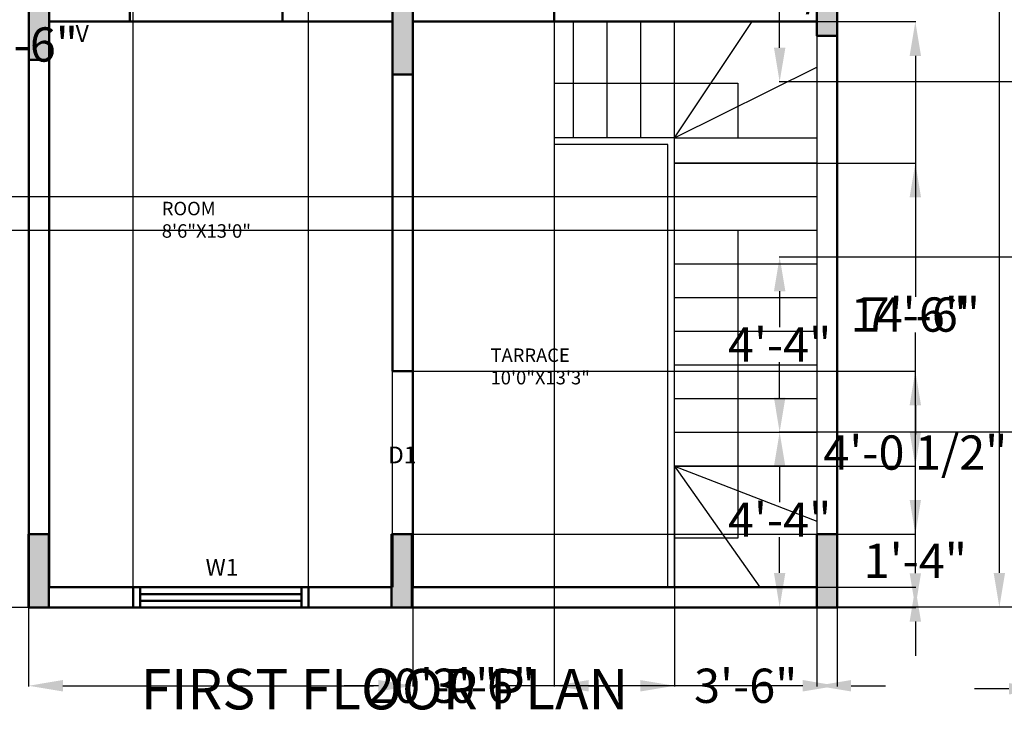
# Model space of a CAD drawing. Units: inches. Extents: x 21 to 3450, y 4 to 2137.
# Tile 3 of 14: x 2513 to 2805, y 1056 to 1261. Entities that reach past the tile are written whole.
import ezdxf

# ---------------------------------------------------------------- set-up
doc = ezdxf.new("R2010")
doc.units = ezdxf.units.IN
doc.header["$MEASUREMENT"] = 0
for name, color, linetype, lineweight in [('A-ANNO-DIMS', 2, 'Continuous', 18), ('A-ANNO-TEXT', 7, 'Continuous', 18), ('A-AREA-IDEN', 3, 'Continuous', 18), ('A-FLOR-STRS', 2, 'Continuous', 25), ('A-WALL', 7, 'Continuous', 50), ('A-WALL-PATT', 8, 'Continuous', 13)]:
    doc.layers.add(name, color=color, linetype=linetype, lineweight=lineweight)
doc.styles.get("Standard").update_dxf_attribs({"font": 'arial.ttf'})
doc.dimstyles.get("Standard").update_dxf_attribs({"dimtxt": 10.18, "dimasz": 10.18, "dimexe": 0.18, "dimexo": 0.0625, "dimgap": 0.09, "dimtad": 0, "dimtih": 1, "dimtoh": 1, "dimdec": 0, "dimzin": 0, "dimdsep": 46, "dimlunit": 3, "dimtxsty": 'Standard', "dimcen": 0.09, "dimadec": 0, "dimazin": 0, "dimtfac": 1, "dimtdec": 0, "dimtofl": 0, "dimtmove": 0, "dimatfit": 3, "dimfxl": 1, "dimtolj": 1, "dimtzin": 0, "dimarcsym": 0})

# ---------------------------------------------------------------- blocks, each defined once
blk = doc.blocks.new('*D8')
at = {"layer": 'A-ANNO-DIMS', "color": 0, "lineweight": -2, "transparency": 16777216}
for p, q in [((2816.85, 1506.81), (2803.73, 1506.81)), ((2803.91, 1496.63), (2803.91, 1302.07)), ((2803.91, 1096.92), (2803.91, 1291.48)), ((2999.5, 1086.74), (2803.73, 1086.74))]:
    blk.add_line(p, q, dxfattribs=at)
at = {"layer": 'A-ANNO-DIMS', "color": 0, "transparency": 16777216}
for points in [[(2802.22, 1496.63), (2805.61, 1496.63), (2803.91, 1506.81)], [(2802.22, 1096.92), (2805.61, 1096.92), (2803.91, 1086.74)]]:
    blk.add_solid(points, dxfattribs=at)
at = {"layer": 'Defpoints', "color": 0, "transparency": 16777216}
for p in [(2816.91, 1506.81), (2803.91, 1086.74), (2999.56, 1086.74)]:
    blk.add_point(p, dxfattribs=at)
at = {"layer": 'A-ANNO-DIMS', "color": 0, "transparency": 16777216, "insert": (2803.91, 1296.77), "char_height": 10.18, "attachment_point": 5}
blk.add_mtext("\\A1;35'", dxfattribs=at)
blk = doc.blocks.new('*D46')
at = {"layer": 'A-ANNO-DIMS', "color": 0, "lineweight": -2, "transparency": 16777216}
for p, q in [((2491.15, 1243.68), (2491.15, 1253.86)), ((2491.15, 1253.86), (2501.33, 1253.86)), ((2461.46, 1233.5), (2491.33, 1233.5)), ((2461.46, 1227.5), (2491.33, 1227.5)), ((2491.15, 1217.32), (2491.15, 1207.14))]:
    blk.add_line(p, q, dxfattribs=at)
at = {"layer": 'A-ANNO-DIMS', "color": 0, "transparency": 16777216}
for points in [[(2489.45, 1243.68), (2492.84, 1243.68), (2491.15, 1233.5)], [(2489.45, 1217.32), (2492.84, 1217.32), (2491.15, 1227.5)]]:
    blk.add_solid(points, dxfattribs=at)
at = {"layer": 'Defpoints', "color": 0, "transparency": 16777216}
for p in [(2461.4, 1233.5), (2491.15, 1233.5), (2461.4, 1227.5)]:
    blk.add_point(p, dxfattribs=at)
at = {"layer": 'A-ANNO-DIMS', "color": 0, "transparency": 16777216, "insert": (2514.95, 1253.86), "char_height": 10.18, "attachment_point": 5}
blk.add_mtext('\\A1;0\'-6"', dxfattribs=at)
blk = doc.blocks.new('*D63')
at = {"layer": 'A-ANNO-DIMS', "color": 0, "lineweight": -2, "transparency": 16777216}
for p, q in [((2417.71, 1189.56), (2417.71, 1521.59)), ((2427.89, 1521.41), (2451.22, 1521.41)), ((2461.4, 1189.56), (2461.4, 1521.59)), ((2461.4, 1521.41), (2471.58, 1521.41))]:
    blk.add_line(p, q, dxfattribs=at)
at = {"layer": 'A-ANNO-DIMS', "color": 0, "transparency": 16777216}
for points in [[(2427.89, 1523.11), (2427.89, 1519.72), (2417.71, 1521.41)], [(2451.22, 1523.11), (2451.22, 1519.72), (2461.4, 1521.41)]]:
    blk.add_solid(points, dxfattribs=at)
at = {"layer": 'Defpoints', "color": 0, "transparency": 16777216}
for p in [(2461.4, 1521.41), (2417.71, 1189.5), (2461.4, 1189.5)]:
    blk.add_point(p, dxfattribs=at)
at = {"layer": 'A-ANNO-DIMS', "color": 0, "transparency": 16777216, "insert": (2497.05, 1521.41), "char_height": 10.18, "attachment_point": 5}
blk.add_mtext('\\A1;3\'-7 1/2"', dxfattribs=at)
blk = doc.blocks.new('*D66')
at = {"layer": 'A-ANNO-DIMS', "color": 0, "lineweight": -2, "transparency": 16777216}
for p, q in [((2515.62, 1086.59), (2515.62, 1063.22)), ((2755.71, 1086.59), (2755.71, 1063.22)), ((2525.8, 1063.4), (2618, 1063.4)), ((2745.53, 1063.4), (2653.32, 1063.4))]:
    blk.add_line(p, q, dxfattribs=at)
at = {"layer": 'A-ANNO-DIMS', "color": 0, "transparency": 16777216}
for points in [[(2525.8, 1065.1), (2525.8, 1061.7), (2515.62, 1063.4)], [(2745.53, 1065.1), (2745.53, 1061.7), (2755.71, 1063.4)]]:
    blk.add_solid(points, dxfattribs=at)
at = {"layer": 'Defpoints', "color": 0, "transparency": 16777216}
for p in [(2515.62, 1086.65), (2755.71, 1086.65), (2755.71, 1063.4)]:
    blk.add_point(p, dxfattribs=at)
at = {"layer": 'A-ANNO-DIMS', "color": 0, "transparency": 16777216, "insert": (2635.66, 1063.4), "char_height": 10.18, "attachment_point": 5}
blk.add_mtext('\\A1;20\'-0"', dxfattribs=at)
blk = doc.blocks.new('*D67')
at = {"layer": 'A-ANNO-DIMS', "color": 0, "lineweight": -2, "transparency": 16777216}
for p, q in [((2515.64, 1506.65), (2492.19, 1506.65)), ((2492.37, 1496.47), (2492.37, 1301.94)), ((2492.37, 1096.83), (2492.37, 1291.36)), ((2515.56, 1086.65), (2492.19, 1086.65))]:
    blk.add_line(p, q, dxfattribs=at)
at = {"layer": 'A-ANNO-DIMS', "color": 0, "transparency": 16777216}
for points in [[(2490.67, 1496.47), (2494.06, 1496.47), (2492.37, 1506.65)], [(2490.67, 1096.83), (2494.06, 1096.83), (2492.37, 1086.65)]]:
    blk.add_solid(points, dxfattribs=at)
at = {"layer": 'Defpoints', "color": 0, "transparency": 16777216}
for p in [(2492.37, 1506.65), (2515.71, 1506.65), (2515.62, 1086.65)]:
    blk.add_point(p, dxfattribs=at)
at = {"layer": 'A-ANNO-DIMS', "color": 0, "transparency": 16777216, "insert": (2492.37, 1296.65), "char_height": 10.18, "attachment_point": 5}
blk.add_mtext('\\A1;35\'-0"', dxfattribs=at)
blk = doc.blocks.new('*D73')
at = {"layer": 'A-ANNO-DIMS', "color": 0, "lineweight": -2, "transparency": 16777216}
for p, q in [((2521.71, 1092.71), (2521.71, 1530.19)), ((2531.89, 1530.01), (2536.53, 1530.01)), ((2546.71, 1092.71), (2546.71, 1530.19)), ((2546.71, 1530.01), (2556.89, 1530.01))]:
    blk.add_line(p, q, dxfattribs=at)
at = {"layer": 'A-ANNO-DIMS', "color": 0, "transparency": 16777216}
for points in [[(2531.89, 1531.71), (2531.89, 1528.31), (2521.71, 1530.01)], [(2536.53, 1531.71), (2536.53, 1528.31), (2546.71, 1530.01)]]:
    blk.add_solid(points, dxfattribs=at)
at = {"layer": 'Defpoints', "color": 0, "transparency": 16777216}
for p in [(2546.71, 1530.01), (2521.71, 1092.65), (2546.71, 1092.65)]:
    blk.add_point(p, dxfattribs=at)
at = {"layer": 'A-ANNO-DIMS', "color": 0, "transparency": 16777216, "insert": (2570.59, 1530.01), "char_height": 10.18, "attachment_point": 5}
blk.add_mtext('\\A1;2\'-1"', dxfattribs=at)
blk = doc.blocks.new('*D74')
at = {"layer": 'A-ANNO-DIMS', "color": 0, "lineweight": -2, "transparency": 16777216}
for p, q in [((2546.71, 1092.71), (2546.71, 1530.19)), ((2556.89, 1530.01), (2558.88, 1530.01)), ((2588.53, 1530.01), (2586.53, 1530.01)), ((2598.71, 1092.71), (2598.71, 1530.19))]:
    blk.add_line(p, q, dxfattribs=at)
at = {"layer": 'A-ANNO-DIMS', "color": 0, "transparency": 16777216}
for points in [[(2556.89, 1531.71), (2556.89, 1528.31), (2546.71, 1530.01)], [(2588.53, 1531.71), (2588.53, 1528.31), (2598.71, 1530.01)]]:
    blk.add_solid(points, dxfattribs=at)
at = {"layer": 'Defpoints', "color": 0, "transparency": 16777216}
for p in [(2598.71, 1530.01), (2546.71, 1092.65), (2598.71, 1092.65)]:
    blk.add_point(p, dxfattribs=at)
at = {"layer": 'A-ANNO-DIMS', "color": 0, "transparency": 16777216, "insert": (2572.71, 1530.01), "char_height": 10.18, "attachment_point": 5}
blk.add_mtext('\\A1;4\'-4"', dxfattribs=at)
blk = doc.blocks.new('*D75')
at = {"layer": 'A-ANNO-DIMS', "color": 0, "lineweight": -2, "transparency": 16777216}
for p, q in [((2598.71, 1092.71), (2598.71, 1530.19)), ((2608.89, 1530.01), (2613.53, 1530.01)), ((2623.71, 1092.71), (2623.71, 1530.19)), ((2623.71, 1530.01), (2633.89, 1530.01))]:
    blk.add_line(p, q, dxfattribs=at)
at = {"layer": 'A-ANNO-DIMS', "color": 0, "transparency": 16777216}
for points in [[(2608.89, 1531.71), (2608.89, 1528.31), (2598.71, 1530.01)], [(2613.53, 1531.71), (2613.53, 1528.31), (2623.71, 1530.01)]]:
    blk.add_solid(points, dxfattribs=at)
at = {"layer": 'Defpoints', "color": 0, "transparency": 16777216}
for p in [(2623.71, 1530.01), (2598.71, 1092.65), (2623.71, 1092.65)]:
    blk.add_point(p, dxfattribs=at)
at = {"layer": 'A-ANNO-DIMS', "color": 0, "transparency": 16777216, "insert": (2647.59, 1530.01), "char_height": 10.18, "attachment_point": 5}
blk.add_mtext('\\A1;2\'-1"', dxfattribs=at)
blk = doc.blocks.new('*D76')
at = {"layer": 'A-ANNO-DIMS', "color": 0, "lineweight": -2, "transparency": 16777216}
for p, q in [((2749.77, 1260.65), (2779.14, 1260.65)), ((2778.96, 1250.47), (2778.96, 1178.94)), ((2778.96, 1096.83), (2778.96, 1168.36)), ((2755.77, 1086.65), (2779.14, 1086.65))]:
    blk.add_line(p, q, dxfattribs=at)
at = {"layer": 'A-ANNO-DIMS', "color": 0, "transparency": 16777216}
for points in [[(2777.26, 1250.47), (2780.65, 1250.47), (2778.96, 1260.65)], [(2777.26, 1096.83), (2780.65, 1096.83), (2778.96, 1086.65)]]:
    blk.add_solid(points, dxfattribs=at)
at = {"layer": 'Defpoints', "color": 0, "transparency": 16777216}
for p in [(2749.71, 1260.65), (2778.96, 1260.65), (2755.71, 1086.65)]:
    blk.add_point(p, dxfattribs=at)
at = {"layer": 'A-ANNO-DIMS', "color": 0, "transparency": 16777216, "insert": (2778.96, 1173.65), "char_height": 10.18, "attachment_point": 5}
blk.add_mtext('\\A1;14\'-6"', dxfattribs=at)
blk = doc.blocks.new('*D77')
at = {"layer": 'A-ANNO-DIMS', "color": 0, "lineweight": -2, "transparency": 16777216}
for p, q in [((2778.96, 1276.83), (2778.96, 1287.01)), ((2778.96, 1287.01), (2789.14, 1287.01)), ((2749.77, 1266.65), (2779.14, 1266.65)), ((2749.77, 1260.65), (2779.14, 1260.65)), ((2778.96, 1250.47), (2778.96, 1240.29))]:
    blk.add_line(p, q, dxfattribs=at)
at = {"layer": 'A-ANNO-DIMS', "color": 0, "transparency": 16777216}
for points in [[(2777.26, 1276.83), (2780.65, 1276.83), (2778.96, 1266.65)], [(2777.26, 1250.47), (2780.65, 1250.47), (2778.96, 1260.65)]]:
    blk.add_solid(points, dxfattribs=at)
at = {"layer": 'Defpoints', "color": 0, "transparency": 16777216}
for p in [(2749.71, 1266.65), (2778.96, 1266.65), (2749.71, 1260.65)]:
    blk.add_point(p, dxfattribs=at)
at = {"layer": 'A-ANNO-DIMS', "color": 0, "transparency": 16777216, "insert": (2802.76, 1287.01), "char_height": 10.18, "attachment_point": 5}
blk.add_mtext('\\A1;0\'-6"', dxfattribs=at)
blk = doc.blocks.new('*D86')
at = {"layer": 'A-ANNO-DIMS', "color": 0, "lineweight": -2, "transparency": 16777216}
for p, q in [((2629.71, 1260.59), (2629.71, 1063.22)), ((2671.75, 1260.59), (2671.75, 1063.22)), ((2619.53, 1063.4), (2609.35, 1063.4)), ((2681.93, 1063.4), (2692.11, 1063.4))]:
    blk.add_line(p, q, dxfattribs=at)
at = {"layer": 'A-ANNO-DIMS', "color": 0, "transparency": 16777216}
for points in [[(2619.53, 1065.1), (2619.53, 1061.7), (2629.71, 1063.4)], [(2681.93, 1065.1), (2681.93, 1061.7), (2671.75, 1063.4)]]:
    blk.add_solid(points, dxfattribs=at)
at = {"layer": 'Defpoints', "color": 0, "transparency": 16777216}
for p in [(2629.71, 1260.65), (2671.75, 1260.65), (2671.75, 1063.4)]:
    blk.add_point(p, dxfattribs=at)
at = {"layer": 'A-ANNO-DIMS', "color": 0, "transparency": 16777216, "insert": (2650.73, 1063.4), "char_height": 10.18, "attachment_point": 5}
blk.add_mtext('\\A1;3\'-6"', dxfattribs=at)
blk = doc.blocks.new('*D87')
at = {"layer": 'A-ANNO-DIMS', "color": 0, "lineweight": -2, "transparency": 16777216}
for p, q in [((2629.77, 1156.88), (2779.14, 1156.88)), ((2778.96, 1146.7), (2778.96, 1138.01)), ((2778.96, 1118.61), (2778.96, 1127.3)), ((2629.49, 1108.43), (2779.14, 1108.43))]:
    blk.add_line(p, q, dxfattribs=at)
at = {"layer": 'A-ANNO-DIMS', "color": 0, "transparency": 16777216}
for points in [[(2777.26, 1146.7), (2780.65, 1146.7), (2778.96, 1156.88)], [(2777.26, 1118.61), (2780.65, 1118.61), (2778.96, 1108.43)]]:
    blk.add_solid(points, dxfattribs=at)
at = {"layer": 'Defpoints', "color": 0, "transparency": 16777216}
for p in [(2629.71, 1156.88), (2778.96, 1156.88), (2629.43, 1108.43)]:
    blk.add_point(p, dxfattribs=at)
at = {"layer": 'A-ANNO-DIMS', "color": 0, "transparency": 16777216, "insert": (2778.96, 1132.66), "char_height": 10.18, "attachment_point": 5}
blk.add_mtext('\\A1;4\'-0 1/2"', dxfattribs=at)
blk = doc.blocks.new('*D88')
at = {"layer": 'A-ANNO-DIMS', "color": 0, "lineweight": -2, "transparency": 16777216}
for p, q in [((2778.96, 1118.61), (2778.96, 1128.79)), ((2629.49, 1108.43), (2779.14, 1108.43)), ((2629.77, 1092.65), (2779.14, 1092.65)), ((2778.96, 1082.47), (2778.96, 1072.29))]:
    blk.add_line(p, q, dxfattribs=at)
at = {"layer": 'A-ANNO-DIMS', "color": 0, "transparency": 16777216}
for points in [[(2777.26, 1118.61), (2780.65, 1118.61), (2778.96, 1108.43)], [(2777.26, 1082.47), (2780.65, 1082.47), (2778.96, 1092.65)]]:
    blk.add_solid(points, dxfattribs=at)
at = {"layer": 'Defpoints', "color": 0, "transparency": 16777216}
for p in [(2629.43, 1108.43), (2778.96, 1108.43), (2629.71, 1092.65)]:
    blk.add_point(p, dxfattribs=at)
at = {"layer": 'A-ANNO-DIMS', "color": 0, "transparency": 16777216, "insert": (2778.96, 1100.54), "char_height": 10.18, "attachment_point": 5}
blk.add_mtext('\\A1;1\'-4"', dxfattribs=at)
blk = doc.blocks.new('*D93')
at = {"layer": 'A-ANNO-DIMS', "color": 0, "lineweight": -2, "transparency": 16777216}
for p, q in [((2707.48, 1128.59), (2707.48, 1063.22)), ((2749.71, 1128.59), (2749.71, 1063.22)), ((2697.3, 1063.4), (2687.12, 1063.4)), ((2759.89, 1063.4), (2770.07, 1063.4))]:
    blk.add_line(p, q, dxfattribs=at)
at = {"layer": 'A-ANNO-DIMS', "color": 0, "transparency": 16777216}
for points in [[(2697.3, 1065.1), (2697.3, 1061.7), (2707.48, 1063.4)], [(2759.89, 1065.1), (2759.89, 1061.7), (2749.71, 1063.4)]]:
    blk.add_solid(points, dxfattribs=at)
at = {"layer": 'Defpoints', "color": 0, "transparency": 16777216}
for p in [(2707.48, 1128.65), (2749.71, 1128.65), (2749.71, 1063.4)]:
    blk.add_point(p, dxfattribs=at)
at = {"layer": 'A-ANNO-DIMS', "color": 0, "transparency": 16777216, "insert": (2728.59, 1063.4), "char_height": 10.18, "attachment_point": 5}
blk.add_mtext('\\A1;3\'-6"', dxfattribs=at)
blk = doc.blocks.new('*D94')
at = {"layer": 'A-ANNO-DIMS', "color": 0, "lineweight": -2, "transparency": 16777216}
for p, q in [((2492.37, 1218.83), (2492.37, 1229.01)), ((2707.42, 1208.65), (2492.19, 1208.65)), ((2707.42, 1198.65), (2492.19, 1198.65)), ((2492.37, 1188.47), (2492.37, 1178.29)), ((2492.37, 1178.29), (2482.19, 1178.29))]:
    blk.add_line(p, q, dxfattribs=at)
at = {"layer": 'A-ANNO-DIMS', "color": 0, "transparency": 16777216}
for points in [[(2490.67, 1218.83), (2494.06, 1218.83), (2492.37, 1208.65)], [(2490.67, 1188.47), (2494.06, 1188.47), (2492.37, 1198.65)]]:
    blk.add_solid(points, dxfattribs=at)
at = {"layer": 'Defpoints', "color": 0, "transparency": 16777216}
for p in [(2707.48, 1208.65), (2492.37, 1198.65), (2707.48, 1198.65)]:
    blk.add_point(p, dxfattribs=at)
at = {"layer": 'A-ANNO-DIMS', "color": 0, "transparency": 16777216, "insert": (2464.61, 1178.29), "char_height": 10.18, "attachment_point": 5}
blk.add_mtext('\\A1;0\'-10"', dxfattribs=at)
blk = doc.blocks.new('*D95')
at = {"layer": 'A-ANNO-DIMS', "color": 0, "lineweight": -2, "transparency": 16777216}
for p, q in [((2707.54, 1218.65), (2779.14, 1218.65)), ((2778.96, 1208.47), (2778.96, 1178.94)), ((2778.96, 1138.83), (2778.96, 1168.36)), ((2707.54, 1128.65), (2779.14, 1128.65))]:
    blk.add_line(p, q, dxfattribs=at)
at = {"layer": 'A-ANNO-DIMS', "color": 0, "transparency": 16777216}
for points in [[(2777.26, 1208.47), (2780.65, 1208.47), (2778.96, 1218.65)], [(2777.26, 1138.83), (2780.65, 1138.83), (2778.96, 1128.65)]]:
    blk.add_solid(points, dxfattribs=at)
at = {"layer": 'Defpoints', "color": 0, "transparency": 16777216}
for p in [(2707.48, 1218.65), (2707.48, 1128.65), (2778.96, 1128.65)]:
    blk.add_point(p, dxfattribs=at)
at = {"layer": 'A-ANNO-DIMS', "color": 0, "transparency": 16777216, "insert": (2778.96, 1173.65), "char_height": 10.18, "attachment_point": 5}
blk.add_mtext('\\A1;7\'-6"', dxfattribs=at)
blk = doc.blocks.new('*D101')
at = {"layer": 'A-ANNO-DIMS', "color": 0, "lineweight": -2, "transparency": 16777216}
for p, q in [((2816.91, 1086.68), (2816.91, 1062.31)), ((2847.91, 1086.68), (2847.91, 1062.31)), ((2806.73, 1062.49), (2796.55, 1062.49)), ((2858.09, 1062.49), (2868.27, 1062.49))]:
    blk.add_line(p, q, dxfattribs=at)
at = {"layer": 'A-ANNO-DIMS', "color": 0, "transparency": 16777216}
for points in [[(2806.73, 1064.19), (2806.73, 1060.8), (2816.91, 1062.49)], [(2858.09, 1064.19), (2858.09, 1060.8), (2847.91, 1062.49)]]:
    blk.add_solid(points, dxfattribs=at)
at = {"layer": 'Defpoints', "color": 0, "transparency": 16777216}
for p in [(2816.91, 1086.74), (2847.91, 1086.74), (2847.91, 1062.49)]:
    blk.add_point(p, dxfattribs=at)
at = {"layer": 'A-ANNO-DIMS', "color": 0, "transparency": 16777216, "insert": (2832.41, 1062.49), "char_height": 10.18, "attachment_point": 5}
blk.add_mtext('\\A1;2\'-7"', dxfattribs=at)
blk = doc.blocks.new('*D114')
at = {"layer": 'A-ANNO-DIMS', "color": 0, "lineweight": -2, "transparency": 16777216}
for p, q in [((2816.85, 1138.74), (2738.48, 1138.74)), ((2738.66, 1128.56), (2738.66, 1117.92)), ((2738.66, 1096.92), (2738.66, 1107.56)), ((2816.85, 1086.74), (2738.48, 1086.74))]:
    blk.add_line(p, q, dxfattribs=at)
at = {"layer": 'A-ANNO-DIMS', "color": 0, "transparency": 16777216}
for points in [[(2736.97, 1128.56), (2740.36, 1128.56), (2738.66, 1138.74)], [(2736.97, 1096.92), (2740.36, 1096.92), (2738.66, 1086.74)]]:
    blk.add_solid(points, dxfattribs=at)
at = {"layer": 'Defpoints', "color": 0, "transparency": 16777216}
for p in [(2738.66, 1138.74), (2816.91, 1138.74), (2816.91, 1086.74)]:
    blk.add_point(p, dxfattribs=at)
at = {"layer": 'A-ANNO-DIMS', "color": 0, "transparency": 16777216, "insert": (2738.66, 1112.74), "char_height": 10.18, "attachment_point": 5}
blk.add_mtext('\\A1;4\'-4"', dxfattribs=at)
blk = doc.blocks.new('*D115')
at = {"layer": 'A-ANNO-DIMS', "color": 0, "lineweight": -2, "transparency": 16777216}
for p, q in [((2816.85, 1190.74), (2738.48, 1190.74)), ((2738.66, 1180.56), (2738.66, 1169.92)), ((2738.66, 1148.92), (2738.66, 1159.56)), ((2816.85, 1138.74), (2738.48, 1138.74))]:
    blk.add_line(p, q, dxfattribs=at)
at = {"layer": 'A-ANNO-DIMS', "color": 0, "transparency": 16777216}
for points in [[(2736.97, 1180.56), (2740.36, 1180.56), (2738.66, 1190.74)], [(2736.97, 1148.92), (2740.36, 1148.92), (2738.66, 1138.74)]]:
    blk.add_solid(points, dxfattribs=at)
at = {"layer": 'Defpoints', "color": 0, "transparency": 16777216}
for p in [(2738.66, 1190.74), (2816.91, 1190.74), (2816.91, 1138.74)]:
    blk.add_point(p, dxfattribs=at)
at = {"layer": 'A-ANNO-DIMS', "color": 0, "transparency": 16777216, "insert": (2738.66, 1164.74), "char_height": 10.18, "attachment_point": 5}
blk.add_mtext('\\A1;4\'-4"', dxfattribs=at)
blk = doc.blocks.new('*D120')
at = {"layer": 'A-ANNO-DIMS', "color": 0, "lineweight": -2, "transparency": 16777216}
for p, q in [((2972.85, 1298.07), (2738.48, 1298.07)), ((2738.66, 1287.89), (2738.66, 1275.76)), ((2738.66, 1252.92), (2738.66, 1265.05)), ((2972.85, 1242.74), (2738.48, 1242.74))]:
    blk.add_line(p, q, dxfattribs=at)
at = {"layer": 'A-ANNO-DIMS', "color": 0, "transparency": 16777216}
for points in [[(2736.97, 1287.89), (2740.36, 1287.89), (2738.66, 1298.07)], [(2736.97, 1252.92), (2740.36, 1252.92), (2738.66, 1242.74)]]:
    blk.add_solid(points, dxfattribs=at)
at = {"layer": 'Defpoints', "color": 0, "transparency": 16777216}
for p in [(2738.66, 1298.07), (2972.91, 1298.07), (2972.91, 1242.74)]:
    blk.add_point(p, dxfattribs=at)
at = {"layer": 'A-ANNO-DIMS', "color": 0, "transparency": 16777216, "insert": (2738.66, 1270.41), "char_height": 10.18, "attachment_point": 5}
blk.add_mtext('\\A1;4\'-7 1/2"', dxfattribs=at)

msp = doc.modelspace()

# ---------------------------------------------------------------- hatches: boundary and pattern name
at = {"layer": 'A-WALL-PATT'}
h = msp.add_hatch(color=256, dxfattribs=at)
h.dxf.hatch_style = 1
h.paths.add_polyline_path([(2521.71, 1506.22), (2515.71, 1506.22), (2515.71, 1484.44), (2521.71, 1484.44)])
h.paths.add_polyline_path([(2618.57, 1506.65), (2596.78, 1506.65), (2596.78, 1500.65), (2618.57, 1500.65)])
h.paths.add_polyline_path([(2755.71, 1506.65), (2749.71, 1506.65), (2749.71, 1484.98), (2755.71, 1484.98)])
h.paths.add_polyline_path([(2755.71, 1403.77), (2749.71, 1403.77), (2749.71, 1381.98), (2755.71, 1381.98)])
h.paths.add_polyline_path([(2602.71, 1408.43), (2596.84, 1408.43), (2596.84, 1386.65), (2602.84, 1386.65), (2602.84, 1392.65), (2602.71, 1392.65)])
h.paths.add_polyline_path([(2755.71, 1278.18), (2749.71, 1278.18), (2749.71, 1256.4), (2755.71, 1256.4)])
h.paths.add_polyline_path([(2521.71, 1271.12), (2515.71, 1271.12), (2515.71, 1249.33), (2521.71, 1249.33)])
h.paths.add_polyline_path([(2521.71, 1408.43), (2515.71, 1408.43), (2515.71, 1386.65), (2521.71, 1386.65)])
h.paths.add_polyline_path([(2629.71, 1266.65), (2623.71, 1266.65), (2623.71, 1244.92), (2629.71, 1244.92)])
h.paths.add_polyline_path([(2521.62, 1108.43), (2515.71, 1108.43), (2515.71, 1086.65), (2521.62, 1086.65)])
h.paths.add_polyline_path([(2629.43, 1108.43), (2623.71, 1108.43), (2623.71, 1092.65), (2623.43, 1086.65), (2629.43, 1086.65)])
h.paths.add_polyline_path([(2755.71, 1108.43), (2749.71, 1108.43), (2749.71, 1086.65), (2755.71, 1086.65)])

# ---------------------------------------------------------------- linework, layer by layer
at = {"layer": 'A-FLOR-STRS'}
for p, q in [((2671.75, 1260.65), (2671.75, 1224.15)), ((2677.48, 1226.15), (2677.48, 1260.65)), ((2687.48, 1226.15), (2687.48, 1260.65)), ((2697.48, 1226.15), (2697.48, 1260.65)), ((2707.48, 1226.15), (2707.48, 1260.65)), ((2707.48, 1226.15), (2730.55, 1260.65)), ((2749.71, 1260.65), (2749.71, 1092.65)), ((2707.48, 1226.15), (2749.71, 1247.13)), ((2671.75, 1242.4), (2726.22, 1242.4)), ((2726.22, 1242.4), (2726.22, 1226.15)), ((2707.48, 1226.15), (2671.75, 1226.15)), ((2707.48, 1092.65), (2707.48, 1226.15)), ((2707.48, 1226.15), (2749.71, 1226.15)), ((2705.48, 1224.15), (2671.75, 1224.15)), ((2705.48, 1092.65), (2705.48, 1224.15)), ((2749.71, 1218.65), (2707.48, 1218.65)), ((2749.71, 1208.65), (2707.48, 1208.65)), ((2749.71, 1208.65), (2707.48, 1208.65)), ((2749.71, 1198.65), (2707.48, 1198.65)), ((2726.22, 1198.65), (2726.22, 1107.22)), ((2749.71, 1188.65), (2707.48, 1188.65)), ((2749.71, 1178.65), (2707.48, 1178.65)), ((2749.71, 1168.65), (2707.48, 1168.65)), ((2749.71, 1158.65), (2707.48, 1158.65)), ((2749.71, 1148.65), (2707.48, 1148.65)), ((2749.71, 1138.65), (2707.48, 1138.65)), ((2749.71, 1128.65), (2707.48, 1128.65)), ((2707.48, 1128.65), (2749.71, 1112.31)), ((2707.48, 1128.65), (2732.8, 1092.65)), ((2726.22, 1107.22), (2707.48, 1107.22))]:
    msp.add_line(p, q, dxfattribs=at)
at = {"layer": 'A-WALL'}
for p, q in [((2515.71, 1086.65), (2515.71, 1506.65)), ((2755.71, 1506.65), (2755.71, 1086.65)), ((2521.71, 1266.65), (2521.71, 1260.65)), ((2545.71, 1266.65), (2545.71, 1260.65)), ((2591.07, 1266.65), (2591.07, 1260.65)), ((2671.71, 1266.65), (2671.71, 1260.57)), ((2521.71, 1092.65), (2521.71, 1260.65)), ((2521.71, 1260.65), (2623.71, 1260.65)), ((2623.71, 1260.65), (2623.71, 1156.88)), ((2629.71, 1260.65), (2629.71, 1092.65)), ((2629.71, 1260.65), (2749.71, 1260.65)), ((2623.71, 1156.88), (2629.71, 1156.88)), ((2623.71, 1108.43), (2623.71, 1092.65)), ((2623.71, 1092.65), (2521.71, 1092.65)), ((2546.71, 1092.65), (2546.71, 1086.65)), ((2548.71, 1092.65), (2548.71, 1086.65)), ((2596.71, 1092.65), (2596.71, 1086.65)), ((2598.71, 1092.65), (2598.71, 1086.65)), ((2749.71, 1092.65), (2629.71, 1092.65)), ((2548.71, 1090.65), (2596.71, 1090.65)), ((2548.71, 1088.65), (2596.71, 1088.65)), ((2755.71, 1086.65), (2515.71, 1086.65))]:
    msp.add_line(p, q, dxfattribs=at)
for points in [[(2749.71, 1278.18), (2755.71, 1278.18), (2755.71, 1256.4), (2749.71, 1256.4)], [(2515.71, 1271.12), (2521.71, 1271.12), (2521.71, 1249.33), (2515.71, 1249.33)], [(2623.71, 1266.7), (2629.71, 1266.7), (2629.71, 1244.92), (2623.71, 1244.92)], [(2515.62, 1108.43), (2521.62, 1108.43), (2521.62, 1086.65), (2515.62, 1086.65)], [(2623.43, 1108.43), (2629.43, 1108.43), (2629.43, 1086.65), (2623.43, 1086.65)], [(2749.71, 1108.43), (2755.71, 1108.43), (2755.71, 1086.65), (2749.71, 1086.65)]]:
    msp.add_lwpolyline(points, close=True, dxfattribs=at)

# ---------------------------------------------------------------- texts
at = {"layer": 'A-ANNO-TEXT', "attachment_point": 1}
for s, width, insert, char_height in [('V', 12.1398, (2529.59, 1259.63), 5), ('D1', 12.1398, (2622.34, 1134.46), 5), ('W1', 12.1398, (2568.18, 1101.07), 5), ('FIRST FLOOR PLAN', 189.6067, (2548.95, 1068.38), 12)]:
    msp.add_mtext_dynamic_manual_height_columns(s, width=width, gutter_width=1, heights=[0], dxfattribs=dict(at, insert=insert, char_height=char_height))
at = {"layer": 'A-AREA-IDEN', "char_height": 4, "attachment_point": 1}
for s, insert in [('ROOM\\P8\'6"X13\'0"', (2555.18, 1207.14)), ('TARRACE\\P10\'0"X13\'3"', (2652.81, 1163.58))]:
    msp.add_mtext_dynamic_manual_height_columns(s, width=50.8458, gutter_width=1, heights=[0], dxfattribs=dict(at, insert=insert))

# ---------------------------------------------------------------- dimensions: what is measured, and where the dimension line sits
at = {"layer": 'A-ANNO-DIMS'}
for base, p1, p2, picture, middle in [((2461.4, 1521.41), (2417.71, 1189.5), (2461.4, 1189.5), '*D63', (2497.05, 1521.41)), ((2546.71, 1530.01), (2521.71, 1092.65), (2546.71, 1092.65), '*D73', (2570.59, 1530.01)), ((2598.71, 1530.01), (2546.71, 1092.65), (2598.71, 1092.65), '*D74', (2572.71, 1530.01)), ((2623.71, 1530.01), (2598.71, 1092.65), (2623.71, 1092.65), '*D75', (2647.59, 1530.01)), ((2671.75, 1063.4), (2629.71, 1260.65), (2671.75, 1260.65), '*D86', (2650.73, 1063.4)), ((2749.71, 1063.4), (2707.48, 1128.65), (2749.71, 1128.65), '*D93', (2728.59, 1063.4)), ((2755.71, 1063.4), (2515.62, 1086.65), (2755.71, 1086.65), '*D66', (2635.66, 1063.4)), ((2847.91, 1062.49), (2816.91, 1086.74), (2847.91, 1086.74), '*D101', (2832.41, 1062.49))]:
    dim = msp.add_linear_dim(base=base, p1=p1, p2=p2, dimstyle='Standard', override={"dimdec": 1, "dimlfac": 1, "dimrnd": 0, "dimzin": 1, "dimdsep": 46, "dimlunit": 4, "dimfrac": 2}, dxfattribs=at)
    dim.commit()
    dim.dimension.update_dxf_attribs({"geometry": picture, "text_midpoint": middle})
for base, p1, p2, override, picture, middle in [((2492.37, 1506.65), (2515.62, 1086.65), (2515.71, 1506.65), {"dimdec": 1, "dimlfac": 1, "dimrnd": 0, "dimzin": 1, "dimdsep": 46, "dimlunit": 4, "dimfrac": 2}, '*D67', (2492.37, 1296.65)), ((2803.91, 1086.74), (2816.91, 1506.81), (2999.56, 1086.74), {"dimclrd": 0, "dimclre": 0, "dimclrt": 0}, '*D8', (2803.91, 1296.77)), ((2738.66, 1298.07), (2972.91, 1242.74), (2972.91, 1298.07), {"dimdec": 1, "dimlfac": 1, "dimrnd": 0, "dimzin": 1, "dimdsep": 46, "dimlunit": 4, "dimfrac": 2}, '*D120', (2738.66, 1270.41)), ((2778.96, 1266.65), (2749.71, 1260.65), (2749.71, 1266.65), {"dimdec": 1, "dimlfac": 1, "dimrnd": 0, "dimzin": 1, "dimdsep": 46, "dimlunit": 4, "dimfrac": 2}, '*D77', (2802.76, 1287.01)), ((2491.15, 1233.5), (2461.4, 1227.5), (2461.4, 1233.5), {"dimdec": 1, "dimlfac": 1, "dimrnd": 0, "dimzin": 1, "dimdsep": 46, "dimlunit": 4, "dimfrac": 2}, '*D46', (2514.95, 1253.86)), ((2778.96, 1260.65), (2755.71, 1086.65), (2749.71, 1260.65), {"dimdec": 1, "dimlfac": 1, "dimrnd": 0, "dimzin": 1, "dimdsep": 46, "dimlunit": 4, "dimfrac": 2}, '*D76', (2778.96, 1173.65)), ((2492.37, 1198.65), (2707.48, 1208.65), (2707.48, 1198.65), {"dimdec": 1, "dimlfac": 1, "dimrnd": 0, "dimzin": 1, "dimdsep": 46, "dimlunit": 4, "dimfrac": 2}, '*D94', (2464.61, 1178.29)), ((2778.96, 1128.65), (2707.48, 1218.65), (2707.48, 1128.65), {"dimdec": 1, "dimlfac": 1, "dimrnd": 0, "dimzin": 1, "dimdsep": 46, "dimlunit": 4, "dimfrac": 2}, '*D95', (2778.96, 1173.65)), ((2738.66, 1190.74), (2816.91, 1138.74), (2816.91, 1190.74), {"dimdec": 1, "dimlfac": 1, "dimrnd": 0, "dimzin": 1, "dimdsep": 46, "dimlunit": 4, "dimfrac": 2}, '*D115', (2738.66, 1164.74)), ((2778.9566, 1156.8812), (2629.4287, 1108.4335), (2629.7066, 1156.8812), {"dimdec": 1, "dimlfac": 1, "dimrnd": 0, "dimzin": 1, "dimdsep": 46, "dimlunit": 4, "dimfrac": 2}, '*D87', (2778.9566, 1132.6574)), ((2738.66, 1138.74), (2816.91, 1086.74), (2816.91, 1138.74), {"dimdec": 1, "dimlfac": 1, "dimrnd": 0, "dimzin": 1, "dimdsep": 46, "dimlunit": 4, "dimfrac": 2}, '*D114', (2738.66, 1112.74)), ((2778.96, 1108.43), (2629.71, 1092.65), (2629.43, 1108.43), {"dimdec": 1, "dimlfac": 1, "dimrnd": 0, "dimzin": 1, "dimdsep": 46, "dimlunit": 4, "dimfrac": 2}, '*D88', (2778.96, 1100.54))]:
    dim = msp.add_linear_dim(base=base, p1=p1, p2=p2, angle=90, dimstyle='Standard', override=override, dxfattribs=at)
    dim.commit()
    dim.dimension.update_dxf_attribs({"geometry": picture, "text_midpoint": middle})

doc.saveas('drawing.dxf')
